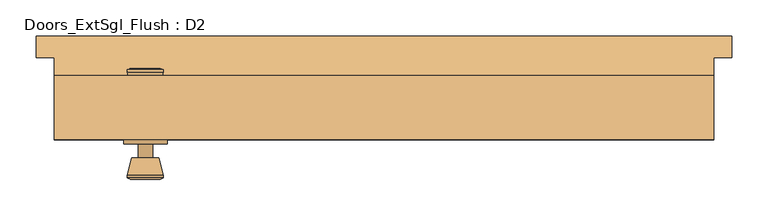
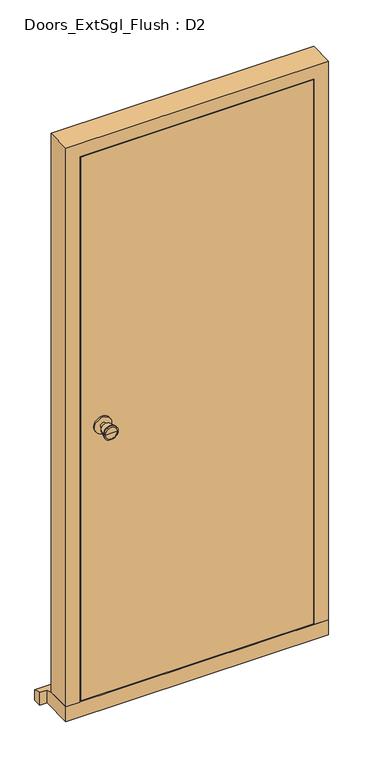
"""IFC4 building model written with IfcOpenShell, lengths in millimetres: door geometry, Doors_ExtSgl_Flush : D2."""

from ifc_helpers import new_model, si_unit, point, frame, frame_2d, origin, place, context, project, spatial, polyline, circle_curve, trimmed, segment, composite_curve, outline, extrude, faceted_brep, source, transform, mapped, element, save
from ifc_brep_helpers import plane_surface, cylinder_surface, revolved_surface, advanced_brep


def doors_extsgl_flush_d2_5e0ff3e2(model_context):
    return source(origin(), model_context, "Body", "SolidModel", [
        advanced_brep(
        [(-330.7, -43.8, 1050.0), (-320.7, -43.8, 1050.0), (-340.7, -43.8, 1050.0), (-310.2241324, -92.8, 1050.0), (-330.7, -92.8, 1050.0), (-351.1758676, -92.8, 1050.0), (-305.7, -90.9721319, 1050.0), (-355.7, -90.9721319, 1050.0), (-305.7, -87.5084537, 1050.0), (-355.7, -87.5084537, 1050.0), (-312.063764, -62.8, 1050.0), (-349.336236, -62.8, 1050.0), (-320.7, -62.8, 1050.0), (-340.7, -62.8, 1050.0)],
        [
            (0, 1),
            (1, 2, circle_curve(frame((-330.7, -43.8, 1050.0), z_axis=(0.0, 1.0, 0.0), x_axis=(-1.0, 0.0, 0.0)), 10.0)),
            (2, 0),
            (2, 1, circle_curve(frame((-330.7, -43.8, 1050.0), z_axis=(0.0, 1.0, 0.0), x_axis=(-1.0, 0.0, 0.0)), 10.0)),
            (3, 4),
            (4, 5),
            (5, 3, circle_curve(frame((-330.7, -92.8, 1050.0), z_axis=(0.0, -1.0, 0.0), x_axis=(-1.0, 0.0, 0.0)), 20.4758676)),
            (3, 5, circle_curve(frame((-330.7, -92.8, 1050.0), z_axis=(0.0, -1.0, 0.0), x_axis=(-1.0, 0.0, 0.0)), 20.4758676)),
            (6, 3),
            (5, 7),
            (7, 6, circle_curve(frame((-330.7, -90.9721319, 1050.0), z_axis=(0.0, -1.0, 0.0), x_axis=(-1.0, 0.0, 0.0)), 25.0)),
            (6, 7, circle_curve(frame((-330.7, -90.9721319, 1050.0), z_axis=(0.0, -1.0, 0.0), x_axis=(-1.0, 0.0, 0.0)), 25.0)),
            (8, 6),
            (7, 9),
            (9, 8, circle_curve(frame((-330.7, -87.5084537, 1050.0), z_axis=(0.0, -1.0, 0.0), x_axis=(-1.0, 0.0, 0.0)), 25.0)),
            (8, 9, circle_curve(frame((-330.7, -87.5084537, 1050.0), z_axis=(0.0, -1.0, 0.0), x_axis=(-1.0, 0.0, 0.0)), 25.0)),
            (10, 8),
            (9, 11),
            (11, 10, circle_curve(frame((-330.7, -62.8, 1050.0), z_axis=(0.0, -1.0, 0.0), x_axis=(-1.0, 0.0, 0.0)), 18.636236)),
            (10, 11, circle_curve(frame((-330.7, -62.8, 1050.0), z_axis=(0.0, -1.0, 0.0), x_axis=(-1.0, 0.0, 0.0)), 18.636236)),
            (12, 10),
            (11, 13),
            (13, 12, circle_curve(frame((-330.7, -62.8, 1050.0), z_axis=(0.0, -1.0, 0.0), x_axis=(-1.0, 0.0, 0.0)), 10.0)),
            (12, 13, circle_curve(frame((-330.7, -62.8, 1050.0), z_axis=(0.0, -1.0, 0.0), x_axis=(-1.0, 0.0, 0.0)), 10.0)),
            (1, 12),
            (13, 2),
        ],
        [
            plane_surface(frame((-330.7, -43.8, 1050.0), z_axis=(0.0, 1.0, 0.0), x_axis=(-1.0, 0.0, 0.0))),
            plane_surface(frame((-330.7, -92.8, 1050.0), z_axis=(0.0, -1.0, 0.0), x_axis=(-1.0, 0.0, 0.0))),
            revolved_surface(polyline([(-351.1758676, -92.8, 1050.0), (-355.7, -90.9721319, 1050.0)]), (-330.7, -43.8, 1050.0), (0.0, 1.0, 0.0)),
            cylinder_surface(frame((-330.7, -43.8, 1050.0), z_axis=(0.0, 1.0, 0.0), x_axis=(-1.0, 0.0, 0.0)), 25.0),
            revolved_surface(polyline([(-355.7, -87.5084537, 1050.0), (-349.336236, -62.8, 1050.0)]), (-330.7, -43.8, 1050.0), (0.0, 1.0, 0.0)),
            plane_surface(frame((-330.7, -62.8, 1050.0), z_axis=(0.0, 1.0, 0.0), x_axis=(-1.0, 0.0, 0.0))),
            cylinder_surface(frame((-330.7, -43.8, 1050.0), z_axis=(0.0, 1.0, 0.0), x_axis=(-1.0, 0.0, 0.0)), 10.0),
        ],
        [
            (0, [[1, 2, 3]]),
            (0, [[-3, 4, -1]]),
            (1, [[5, 6, 7]]),
            (1, [[-6, -5, 8]]),
            (2, [[9, -7, 10, 11]]),
            (2, [[-10, -8, -9, 12]]),
            (3, [[13, -11, 14, 15]]),
            (3, [[-14, -12, -13, 16]]),
            (4, [[17, -15, 18, 19]]),
            (4, [[-18, -16, -17, 20]]),
            (5, [[21, -19, 22, 23]]),
            (5, [[-22, -20, -21, 24]]),
            (6, [[25, -23, 26, -2]]),
            (6, [[-26, -24, -25, -4]]),
        ],
    ),
        extrude(outline(composite_curve([segment(trimmed(circle_curve(frame_2d((1050.0, -330.7)), 30.0), [point((1050.0, -360.7))], [point((1050.0, -300.7))], False, "CARTESIAN"), True, "CONTINUOUS"), segment(trimmed(circle_curve(frame_2d((1050.0, -330.7)), 30.0), [point((1050.0, -300.7))], [point((1050.0, -360.7))], False, "CARTESIAN"), True, "CONTINUOUS")], self_intersect=False)), frame((0.0, -43.8, 0.0), z_axis=(0.0, 1.0, 0.0), x_axis=(0.0, 0.0, 1.0)), (0.0, 0.0, 1.0), 6.0),
        advanced_brep(
        [(-330.7, 12.2, 1050.0), (-340.7, 12.2, 1050.0), (-320.7, 12.2, 1050.0), (-310.2241324, 61.2, 1050.0), (-351.1758676, 61.2, 1050.0), (-330.7, 61.2, 1050.0), (-305.7, 59.3721319, 1050.0), (-355.7, 59.3721319, 1050.0), (-305.7, 55.9084537, 1050.0), (-355.7, 55.9084537, 1050.0), (-312.063764, 31.2, 1050.0), (-349.336236, 31.2, 1050.0), (-320.7, 31.2, 1050.0), (-340.7, 31.2, 1050.0)],
        [
            (0, 1),
            (1, 2, circle_curve(frame((-330.7, 12.2, 1050.0), z_axis=(0.0, -1.0, 0.0), x_axis=(-1.0, 0.0, 0.0)), 10.0)),
            (2, 0),
            (2, 1, circle_curve(frame((-330.7, 12.2, 1050.0), z_axis=(0.0, -1.0, 0.0), x_axis=(-1.0, 0.0, 0.0)), 10.0)),
            (3, 4, circle_curve(frame((-330.7, 61.2, 1050.0), z_axis=(0.0, 1.0, 0.0), x_axis=(-1.0, 0.0, 0.0)), 20.4758676)),
            (4, 5),
            (5, 3),
            (4, 3, circle_curve(frame((-330.7, 61.2, 1050.0), z_axis=(0.0, 1.0, 0.0), x_axis=(-1.0, 0.0, 0.0)), 20.4758676)),
            (6, 7, circle_curve(frame((-330.7, 59.3721319, 1050.0), z_axis=(0.0, 1.0, 0.0), x_axis=(-1.0, 0.0, 0.0)), 25.0)),
            (7, 4),
            (3, 6),
            (7, 6, circle_curve(frame((-330.7, 59.3721319, 1050.0), z_axis=(0.0, 1.0, 0.0), x_axis=(-1.0, 0.0, 0.0)), 25.0)),
            (8, 9, circle_curve(frame((-330.7, 55.9084537, 1050.0), z_axis=(0.0, 1.0, 0.0), x_axis=(-1.0, 0.0, 0.0)), 25.0)),
            (9, 7),
            (6, 8),
            (9, 8, circle_curve(frame((-330.7, 55.9084537, 1050.0), z_axis=(0.0, 1.0, 0.0), x_axis=(-1.0, 0.0, 0.0)), 25.0)),
            (10, 11, circle_curve(frame((-330.7, 31.2, 1050.0), z_axis=(0.0, 1.0, 0.0), x_axis=(-1.0, 0.0, 0.0)), 18.636236)),
            (11, 9),
            (8, 10),
            (11, 10, circle_curve(frame((-330.7, 31.2, 1050.0), z_axis=(0.0, 1.0, 0.0), x_axis=(-1.0, 0.0, 0.0)), 18.636236)),
            (12, 13, circle_curve(frame((-330.7, 31.2, 1050.0), z_axis=(0.0, 1.0, 0.0), x_axis=(-1.0, 0.0, 0.0)), 10.0)),
            (13, 11),
            (10, 12),
            (13, 12, circle_curve(frame((-330.7, 31.2, 1050.0), z_axis=(0.0, 1.0, 0.0), x_axis=(-1.0, 0.0, 0.0)), 10.0)),
            (1, 13),
            (12, 2),
        ],
        [
            plane_surface(frame((-330.7, 12.2, 1050.0), z_axis=(0.0, -1.0, 0.0), x_axis=(-1.0, 0.0, 0.0))),
            plane_surface(frame((-330.7, 61.2, 1050.0), z_axis=(0.0, 1.0, 0.0), x_axis=(-1.0, 0.0, 0.0))),
            revolved_surface(polyline([(-351.1758676, 61.2, 1050.0), (-355.7, 59.3721319, 1050.0)]), (-330.7, 12.2, 1050.0), (0.0, -1.0, 0.0)),
            cylinder_surface(frame((-330.7, 12.2, 1050.0), z_axis=(0.0, -1.0, 0.0), x_axis=(-1.0, 0.0, 0.0)), 25.0),
            revolved_surface(polyline([(-355.7, 55.9084537, 1050.0), (-349.336236, 31.2, 1050.0)]), (-330.7, 12.2, 1050.0), (0.0, -1.0, 0.0)),
            plane_surface(frame((-330.7, 31.2, 1050.0), z_axis=(0.0, -1.0, 0.0), x_axis=(-1.0, 0.0, 0.0))),
            cylinder_surface(frame((-330.7, 12.2, 1050.0), z_axis=(0.0, -1.0, 0.0), x_axis=(-1.0, 0.0, 0.0)), 10.0),
        ],
        [
            (0, [[1, 2, 3]]),
            (0, [[-3, 4, -1]]),
            (1, [[5, 6, 7]]),
            (1, [[8, -7, -6]]),
            (2, [[9, 10, -5, 11]]),
            (2, [[12, -11, -8, -10]]),
            (3, [[13, 14, -9, 15]]),
            (3, [[16, -15, -12, -14]]),
            (4, [[17, 18, -13, 19]]),
            (4, [[20, -19, -16, -18]]),
            (5, [[21, 22, -17, 23]]),
            (5, [[24, -23, -20, -22]]),
            (6, [[-2, 25, -21, 26]]),
            (6, [[-4, -26, -24, -25]]),
        ],
    ),
        extrude(outline(composite_curve([segment(trimmed(circle_curve(frame_2d((1050.0, -330.7)), 30.0), [point((1050.0, -360.7))], [point((1050.0, -300.7))], False, "CARTESIAN"), True, "CONTINUOUS"), segment(trimmed(circle_curve(frame_2d((1050.0, -330.7)), 30.0), [point((1050.0, -300.7))], [point((1050.0, -360.7))], False, "CARTESIAN"), True, "CONTINUOUS")], self_intersect=False)), frame((0.0, 6.2, 0.0), z_axis=(0.0, 1.0, 0.0), x_axis=(0.0, 0.0, 1.0)), (0.0, 0.0, 1.0), 6.0),
        faceted_brep([(386.7, 51.2, 54.5), (457.2, 51.2, 54.5), (457.2, -37.8, 54.5), (408.7, -37.8, 54.5), (408.7, 9.2, 54.5), (386.7, 9.2, 54.5), (386.7, 51.2, 2039.5), (-386.7, 51.2, 2039.5), (-386.7, 51.2, 54.5), (-457.2, 51.2, 54.5), (-457.2, 51.2, 2110.0), (457.2, 51.2, 2110.0), (457.2, -37.8, 2110.0), (-457.2, -37.8, 2110.0), (-457.2, -37.8, 54.5), (-408.7, -37.8, 54.5), (-408.7, -37.8, 2061.5), (408.7, -37.8, 2061.5), (408.7, 9.2, 2061.5), (-408.7, 9.2, 2061.5), (-408.7, 9.2, 54.5), (-386.7, 9.2, 54.5), (-386.7, 9.2, 2039.5), (386.7, 9.2, 2039.5)], [[[0, 1, 2, 3, 4, 5]], [[1, 0, 6, 7, 8, 9, 10, 11]], [[2, 1, 11, 12]], [[3, 2, 12, 13, 14, 15, 16, 17]], [[4, 3, 17, 18]], [[5, 4, 18, 19, 20, 21, 22, 23]], [[0, 5, 23, 6]], [[7, 22, 21, 8]], [[8, 21, 20, 15, 14, 9]], [[13, 10, 9, 14]], [[19, 16, 15, 20]], [[12, 11, 10, 13]], [[18, 17, 16, 19]], [[6, 23, 22, 7]]]),
        extrude(outline(polyline([(405.7, -37.8), (-406.6250294, -37.8), (-406.6250294, 6.2), (405.7, 6.2), (405.7, -37.8)])), frame((0.0, 0.0, 58.5), z_axis=(0.0, 0.0, 1.0), x_axis=(1.0, 0.0, 0.0)), (0.0, 0.0, 1.0), 2000.0),
        faceted_brep([(482.2, 106.2, 0.0), (482.2, 106.2, 38.5947221), (482.2, 76.2, 47.2703282), (482.2, 76.2, 0.0), (-482.2, 106.2, 38.5947221), (-482.2, 106.2, 0.0), (-482.2, 76.2, 0.0), (-482.2, 76.2, 47.2703282), (457.2, 76.2, 0.0), (457.2, -37.8, 0.0), (-457.2, -37.8, 0.0), (-457.2, 76.2, 0.0), (-457.2, 76.2, 47.2703282), (-457.2, 51.2, 54.5), (457.2, 51.2, 54.5), (457.2, 76.2, 47.2703282), (-457.2, -37.8, 54.5), (457.2, -37.8, 54.5)], [[[0, 1, 2, 3]], [[4, 5, 6, 7]], [[5, 0, 3, 8, 9, 10, 11, 6]], [[1, 0, 5, 4]], [[1, 4, 7, 12, 13, 14, 15, 2]], [[13, 16, 17, 14]], [[16, 10, 9, 17]], [[12, 11, 10, 16, 13]], [[11, 12, 7, 6]], [[8, 15, 14, 17, 9]], [[15, 8, 3, 2]]]),
    ])


if __name__ == "__main__":
    model = new_model("IFC4")
    model_context = context("Model", 3, world=origin())
    ifc_project = project(units=[si_unit("LENGTHUNIT", "METRE", prefix="MILLI")], contexts=[model_context])
    site = spatial("IfcSite", under=ifc_project)
    building = spatial("IfcBuilding", under=site)
    placement = place(None, origin())
    doors_extsgl_flush_d2_shape = doors_extsgl_flush_d2_5e0ff3e2(model_context)
    element("IfcDoor", 1, ObjectType="Doors_ExtSgl_Flush : D2", at=placement, inside=building, context=model_context, shape_type="MappedRepresentation", body=[
        mapped(doors_extsgl_flush_d2_shape, transform((0.0, 0.0, 0.0), x_axis=(1.0, 0.0, 0.0), y_axis=(0.0, 1.0, 0.0), z_axis=(0.0, 0.0, 1.0))),
    ])
    save(model, "model.ifc")

# Revit data of these elements
# Type "Doors_ExtSgl_Flush : D2"
#   Type Mark = "50"
#   Type Comments = "External Single"
#   Operation = "SingleSwingRight"
#   Construction Type Id = "MDOOR"
#   Keynote = "L20"
#   Analytic Construction = "Metal"
#   Wrap Layers (Int) from Ext = 177.5 mm
#   Wrap Layers (Ext) from Ext = 102.5 mm
#   Thickness = 44 mm
#   Rough Width = 914.4 mm
#   Rough Height = 2110 mm
#   O/A Frame Width = 64 mm
#   Heat Transfer Coefficient (U) = 3.7021 W/(m²·K)
#   Handle Z Distance = 1050 mm
#   FrameWidth = 42 mm
#   FrameOffset - External = 25 mm
#   FrameDepth = 89 mm
#   Door Panel Width = 811.4 mm
#   Door Panel Thickness = 44 mm
#   Door Panel Height = 2000 mm
#   Cill Thickness = 54.5 mm
#   Cill Projection = 30 mm
#   Handle X Distance = 75 mm
#   Height = 2110 mm
#   Structural Tolerance = 6.5 mm
#   Tolerance = 3 mm
#   Undercut = 4 mm
#   Width = 914.4 mm
#   Cill Extension = 25 mm
#   Cavity Closer Width = 50 mm
#   Cavity Closer Offset from Ext = 102.5 mm
#   Cavity Closer Depth = 85 mm
#   Vis - Ironmongery = yes
#   Vis - Cavity Closers = yes
#   Define Thermal Properties by = 1
#   Function = 1
#   Material Door = Door - Panel
#   Material Frame = Door - Frame/Mullion
#   Material Ironmongery = Door - Handle
#   Visual Light Transmittance = 0
#   Solar Heat Gain Coefficient = 0
#   Wall Closure = (empty or 0)
# Element 1 (IfcDoor, "Doors_ExtSgl_Flush : D2")
#   Materials on its faces: "Door - Handle", "Door - Frame/Mullion", "Door - Panel"
# Materials
#   "Door - Panel": class "Wood", colour RGB 210 159 95, transparency 0, Keynote = "L20", Cost = 0
#   "Door - Frame/Mullion": class "Wood", colour RGB 212 179 113, transparency 0, Keynote = "L20", Cost = 0
#   "Door - Handle": colour RGB 0 0 0, transparency 0, Keynote = "P21", Cost = 0
